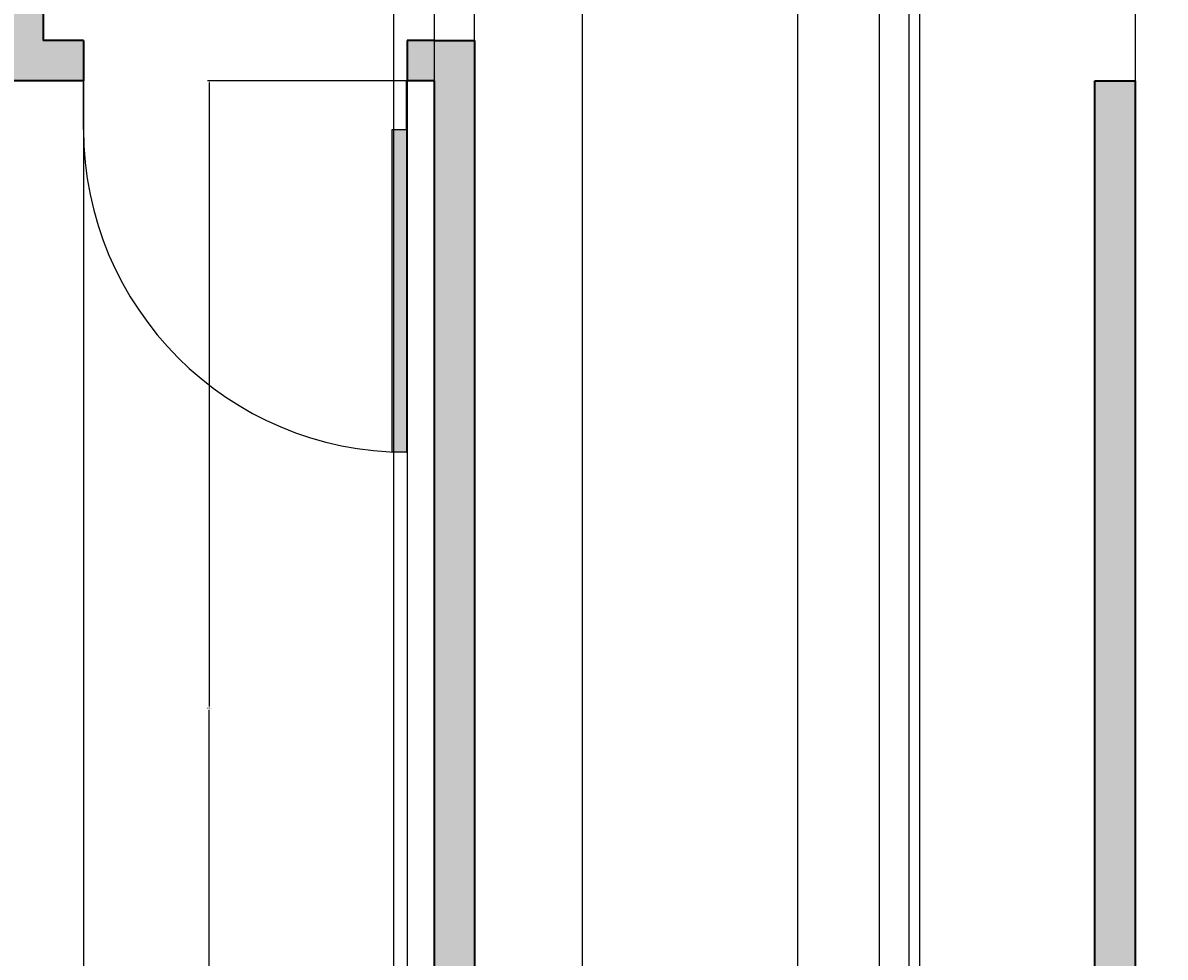
# Model space of a CAD drawing. Units: inches. Extents: x 1434 to 1845, y 1483 to 2014.
# Tile 3 of 11: x 1571 to 1698, y 1633 to 1737. Entities that reach past the tile are written whole.
import ezdxf

# ---------------------------------------------------------------- set-up
doc = ezdxf.new("R2010")
doc.units = ezdxf.units.IN
for name, color, linetype, lineweight in [('A-ANNO-DIMS', 2, 'Continuous', 18), ('A-DOOR', 3, 'Continuous', 25), ('A-WALL', 7, 'Continuous', 35), ('A-WALL-PATT', 8, 'Continuous', 13)]:
    doc.layers.add(name, color=color, linetype=linetype, lineweight=lineweight)
doc.layers.add('A-DOOR-PATT', color=39, linetype='Continuous', lineweight=13, true_color=0x58382b)
doc.styles.get("Standard").update_dxf_attribs({"font": 'arial.ttf'})
doc.dimstyles.get("Standard").update_dxf_attribs({"dimtxt": 0.18, "dimasz": 0.18, "dimexe": 0.18, "dimexo": 0.0625, "dimgap": 0.09, "dimtad": 0, "dimtih": 1, "dimtoh": 1, "dimdec": 4, "dimzin": 0, "dimdsep": 46, "dimtxsty": 'Standard', "dimcen": 0.09, "dimadec": 0, "dimazin": 0, "dimtfac": 1, "dimtdec": 4, "dimtofl": 0, "dimtmove": 0, "dimatfit": 3, "dimfxl": 1, "dimtolj": 1, "dimtzin": 0, "dimarcsym": 0})

# ---------------------------------------------------------------- blocks, each defined once
blk = doc.blocks.new('*U4')
for p, q in [((-40, 0), (-40, 6)), ((0, 0), (0, 6))]:
    blk.add_line(p, q)
blk.add_lwpolyline([(0, 0), (0, -40), (-1.75, -40), (-1.75, 0)], close=True)
blk.add_arc((0, 0), 40, 180, 270)
blk = doc.blocks.new('*D56')
at = {"layer": 'A-ANNO-DIMS', "color": 0, "lineweight": -2, "transparency": 16777216}
for p, q in [((1472.97, 1974.79), (1472.97, 1483.15)), ((1612.47, 1974.79), (1612.47, 1483.15)), ((1473.15, 1483.33), (1542.34, 1483.33)), ((1612.29, 1483.33), (1543.11, 1483.33))]:
    blk.add_line(p, q, dxfattribs=at)
at = {"layer": 'A-ANNO-DIMS', "color": 0, "transparency": 16777216}
for points in [[(1473.15, 1483.36), (1473.15, 1483.3), (1472.97, 1483.33)], [(1612.29, 1483.36), (1612.29, 1483.3), (1612.47, 1483.33)]]:
    blk.add_solid(points, dxfattribs=at)
at = {"layer": 'Defpoints', "color": 0, "transparency": 16777216}
for p in [(1472.97, 1974.86), (1612.47, 1974.86), (1612.47, 1483.33)]:
    blk.add_point(p, dxfattribs=at)
at = {"layer": 'A-ANNO-DIMS', "color": 0, "transparency": 16777216, "insert": (1542.72, 1483.33), "char_height": 0.18, "attachment_point": 5}
blk.add_mtext('\\A1;139.5', dxfattribs=at)
blk = doc.blocks.new('*D57')
at = {"layer": 'A-ANNO-DIMS', "color": 0, "lineweight": -2, "transparency": 16777216}
for p, q in [((1616.97, 1974.79), (1616.97, 1483.15)), ((1666.47, 1974.79), (1666.47, 1483.15)), ((1617.15, 1483.33), (1641.4, 1483.33)), ((1666.29, 1483.33), (1642.05, 1483.33))]:
    blk.add_line(p, q, dxfattribs=at)
at = {"layer": 'A-ANNO-DIMS', "color": 0, "transparency": 16777216}
for points in [[(1617.15, 1483.36), (1617.15, 1483.3), (1616.97, 1483.33)], [(1666.29, 1483.36), (1666.29, 1483.3), (1666.47, 1483.33)]]:
    blk.add_solid(points, dxfattribs=at)
at = {"layer": 'Defpoints', "color": 0, "transparency": 16777216}
for p in [(1616.97, 1974.86), (1666.47, 1974.86), (1666.47, 1483.33)]:
    blk.add_point(p, dxfattribs=at)
at = {"layer": 'A-ANNO-DIMS', "color": 0, "transparency": 16777216, "insert": (1641.72, 1483.33), "char_height": 0.18, "attachment_point": 5}
blk.add_mtext('\\A1;49.5', dxfattribs=at)
blk = doc.blocks.new('*D58')
at = {"layer": 'A-ANNO-DIMS', "color": 0, "lineweight": -2, "transparency": 16777216}
for p, q in [((1670.97, 1974.79), (1670.97, 1483.15)), ((1810.47, 1974.79), (1810.47, 1483.15)), ((1671.15, 1483.33), (1740.34, 1483.33)), ((1810.29, 1483.33), (1741.11, 1483.33))]:
    blk.add_line(p, q, dxfattribs=at)
at = {"layer": 'A-ANNO-DIMS', "color": 0, "transparency": 16777216}
for points in [[(1671.15, 1483.36), (1671.15, 1483.3), (1670.97, 1483.33)], [(1810.29, 1483.36), (1810.29, 1483.3), (1810.47, 1483.33)]]:
    blk.add_solid(points, dxfattribs=at)
at = {"layer": 'Defpoints', "color": 0, "transparency": 16777216}
for p in [(1670.97, 1974.86), (1810.47, 1974.86), (1810.47, 1483.33)]:
    blk.add_point(p, dxfattribs=at)
at = {"layer": 'A-ANNO-DIMS', "color": 0, "transparency": 16777216, "insert": (1740.72, 1483.33), "char_height": 0.18, "attachment_point": 5}
blk.add_mtext('\\A1;139.5', dxfattribs=at)
blk = doc.blocks.new('*D65')
at = {"layer": 'A-ANNO-DIMS', "color": 0, "lineweight": -2, "transparency": 16777216}
for p, q in [((1616.91, 1730.36), (1591.77, 1730.36)), ((1591.95, 1730.18), (1591.95, 1660.79)), ((1591.95, 1591.04), (1591.95, 1660.42)), ((1616.91, 1590.86), (1591.77, 1590.86))]:
    blk.add_line(p, q, dxfattribs=at)
at = {"layer": 'A-ANNO-DIMS', "color": 0, "transparency": 16777216}
for points in [[(1591.92, 1730.18), (1591.98, 1730.18), (1591.95, 1730.36)], [(1591.92, 1591.04), (1591.98, 1591.04), (1591.95, 1590.86)]]:
    blk.add_solid(points, dxfattribs=at)
at = {"layer": 'Defpoints', "color": 0, "transparency": 16777216}
for p in [(1591.95, 1730.36), (1616.97, 1730.36), (1616.97, 1590.86)]:
    blk.add_point(p, dxfattribs=at)
at = {"layer": 'A-ANNO-DIMS', "color": 0, "transparency": 16777216, "insert": (1591.95, 1660.61), "char_height": 0.18, "attachment_point": 5}
blk.add_mtext('\\A1;139.5', dxfattribs=at)
blk = doc.blocks.new('*D67')
at = {"layer": 'A-ANNO-DIMS', "color": 0, "lineweight": -2, "transparency": 16777216}
for p, q in [((1694.97, 1517.42), (1694.97, 2013.56)), ((1695.15, 2013.38), (1752.34, 2013.38)), ((1810.29, 2013.38), (1753.11, 2013.38)), ((1810.47, 1517.42), (1810.47, 2013.56))]:
    blk.add_line(p, q, dxfattribs=at)
at = {"layer": 'A-ANNO-DIMS', "color": 0, "transparency": 16777216}
for points in [[(1695.15, 2013.41), (1695.15, 2013.35), (1694.97, 2013.38)], [(1810.29, 2013.41), (1810.29, 2013.35), (1810.47, 2013.38)]]:
    blk.add_solid(points, dxfattribs=at)
at = {"layer": 'Defpoints', "color": 0, "transparency": 16777216}
for p in [(1810.47, 2013.38), (1694.97, 1517.36), (1810.47, 1517.36)]:
    blk.add_point(p, dxfattribs=at)
at = {"layer": 'A-ANNO-DIMS', "color": 0, "transparency": 16777216, "insert": (1752.72, 2013.38), "char_height": 0.18, "attachment_point": 5}
blk.add_mtext('\\A1;115.5', dxfattribs=at)
blk = doc.blocks.new('*D71')
at = {"layer": 'A-ANNO-DIMS', "color": 0, "lineweight": -2, "transparency": 16777216}
for p, q in [((1633.47, 1508.42), (1633.47, 2013.56)), ((1633.65, 2013.38), (1651.25, 2013.38)), ((1669.64, 2013.38), (1652.04, 2013.38)), ((1669.82, 1508.42), (1669.82, 2013.56))]:
    blk.add_line(p, q, dxfattribs=at)
at = {"layer": 'A-ANNO-DIMS', "color": 0, "transparency": 16777216}
for points in [[(1633.65, 2013.41), (1633.65, 2013.35), (1633.47, 2013.38)], [(1669.64, 2013.41), (1669.64, 2013.35), (1669.82, 2013.38)]]:
    blk.add_solid(points, dxfattribs=at)
at = {"layer": 'Defpoints', "color": 0, "transparency": 16777216}
for p in [(1669.82, 2013.38), (1633.47, 1508.36), (1669.82, 1508.36)]:
    blk.add_point(p, dxfattribs=at)
at = {"layer": 'A-ANNO-DIMS', "color": 0, "transparency": 16777216, "insert": (1651.65, 2013.38), "char_height": 0.18, "attachment_point": 5}
blk.add_mtext('\\A1;36.35', dxfattribs=at)
blk = doc.blocks.new('*D72')
at = {"layer": 'A-ANNO-DIMS', "color": 0, "lineweight": -2, "transparency": 16777216}
for p, q in [((1621.47, 1517.42), (1621.47, 2013.56)), ((1621.65, 2013.38), (1627.26, 2013.38)), ((1633.29, 2013.38), (1627.68, 2013.38)), ((1633.47, 1517.42), (1633.47, 2013.56))]:
    blk.add_line(p, q, dxfattribs=at)
at = {"layer": 'A-ANNO-DIMS', "color": 0, "transparency": 16777216}
for points in [[(1621.65, 2013.41), (1621.65, 2013.35), (1621.47, 2013.38)], [(1633.29, 2013.41), (1633.29, 2013.35), (1633.47, 2013.38)]]:
    blk.add_solid(points, dxfattribs=at)
at = {"layer": 'Defpoints', "color": 0, "transparency": 16777216}
for p in [(1633.47, 2013.38), (1621.47, 1517.36), (1633.47, 1517.36)]:
    blk.add_point(p, dxfattribs=at)
at = {"layer": 'A-ANNO-DIMS', "color": 0, "transparency": 16777216, "insert": (1627.47, 2013.38), "char_height": 0.18, "attachment_point": 5}
blk.add_mtext('\\A1;12', dxfattribs=at)
blk = doc.blocks.new('*D73')
at = {"layer": 'A-ANNO-DIMS', "color": 0, "lineweight": -2, "transparency": 16777216}
for p, q in [((1577.97, 1730.29), (1577.97, 1483.15)), ((1613.97, 1730.29), (1613.97, 1483.15)), ((1578.15, 1483.33), (1595.76, 1483.33)), ((1613.79, 1483.33), (1596.19, 1483.33))]:
    blk.add_line(p, q, dxfattribs=at)
at = {"layer": 'A-ANNO-DIMS', "color": 0, "transparency": 16777216}
for points in [[(1578.15, 1483.36), (1578.15, 1483.3), (1577.97, 1483.33)], [(1613.79, 1483.36), (1613.79, 1483.3), (1613.97, 1483.33)]]:
    blk.add_solid(points, dxfattribs=at)
at = {"layer": 'Defpoints', "color": 0, "transparency": 16777216}
for p in [(1577.97, 1730.36), (1613.97, 1730.36), (1613.97, 1483.33)]:
    blk.add_point(p, dxfattribs=at)
at = {"layer": 'A-ANNO-DIMS', "color": 0, "transparency": 16777216, "insert": (1595.97, 1483.33), "char_height": 0.18, "attachment_point": 5}
blk.add_mtext('\\A1;36', dxfattribs=at)
blk = doc.blocks.new('*D81')
at = {"layer": 'A-ANNO-DIMS', "color": 0, "lineweight": -2, "transparency": 16777216}
for p, q in [((1690.47, 1730.29), (1690.47, 1483.15)), ((1694.97, 1730.29), (1694.97, 1483.15)), ((1690.65, 1483.33), (1692.47, 1483.33)), ((1694.79, 1483.33), (1692.98, 1483.33))]:
    blk.add_line(p, q, dxfattribs=at)
at = {"layer": 'A-ANNO-DIMS', "color": 0, "transparency": 16777216}
for points in [[(1690.65, 1483.36), (1690.65, 1483.3), (1690.47, 1483.33)], [(1694.79, 1483.36), (1694.79, 1483.3), (1694.97, 1483.33)]]:
    blk.add_solid(points, dxfattribs=at)
at = {"layer": 'Defpoints', "color": 0, "transparency": 16777216}
for p in [(1690.47, 1730.36), (1694.97, 1730.36), (1694.97, 1483.33)]:
    blk.add_point(p, dxfattribs=at)
at = {"layer": 'A-ANNO-DIMS', "color": 0, "transparency": 16777216, "insert": (1692.72, 1483.33), "char_height": 0.18, "attachment_point": 5}
blk.add_mtext('\\A1;4.5', dxfattribs=at)
blk = doc.blocks.new('*D86')
at = {"layer": 'A-ANNO-DIMS', "color": 0, "lineweight": -2, "transparency": 16777216}
for p, q in [((1657.38, 1854.66), (1657.38, 1483.15)), ((1666.47, 1854.79), (1666.47, 1483.15)), ((1657.56, 1483.33), (1661.53, 1483.33)), ((1666.29, 1483.33), (1662.32, 1483.33))]:
    blk.add_line(p, q, dxfattribs=at)
at = {"layer": 'A-ANNO-DIMS', "color": 0, "transparency": 16777216}
for points in [[(1657.56, 1483.36), (1657.56, 1483.3), (1657.38, 1483.33)], [(1666.29, 1483.36), (1666.29, 1483.3), (1666.47, 1483.33)]]:
    blk.add_solid(points, dxfattribs=at)
at = {"layer": 'Defpoints', "color": 0, "transparency": 16777216}
for p in [(1657.38, 1854.72), (1666.47, 1854.86), (1657.38, 1483.33)]:
    blk.add_point(p, dxfattribs=at)
at = {"layer": 'A-ANNO-DIMS', "color": 0, "transparency": 16777216, "insert": (1661.93, 1483.33), "char_height": 0.18, "attachment_point": 5}
blk.add_mtext('\\A1;9.096', dxfattribs=at)

msp = doc.modelspace()

# ---------------------------------------------------------------- hatches: boundary and pattern name
at = {"layer": 'A-DOOR-PATT'}
h = msp.add_hatch(color=256, dxfattribs=at)
h.dxf.hatch_style = 1
h.paths.add_polyline_path([(1611.5864, 1583.2737), (1575.6681, 1583.2737, 0.01094143), (1575.7025, 1581.7022), (1611.5864, 1581.7022)])
h.paths.add_polyline_path([(1621.4742, 1547.3553), (1616.9742, 1547.3553), (1616.9742, 1544.3553), (1621.4742, 1544.3553)])
h.paths.add_polyline_path([(1635.0456, 1558.627, 0.01094143), (1633.4742, 1558.6614), (1633.4742, 1522.7431), (1635.0456, 1522.7431)])
h.paths.add_polyline_path([(1633.4742, 1517.3553), (1630.4742, 1517.3553), (1630.4742, 1508.3553), (1633.4742, 1508.3553)])
h.paths.add_polyline_path([(1672.8212, 1517.3553), (1669.8212, 1517.3553), (1669.8212, 1508.3553), (1672.8212, 1508.3553)])
h.paths.add_polyline_path([(1613.8925, 1724.9676), (1612.3211, 1724.9676), (1612.3211, 1689.0836, 0.01094143), (1613.8925, 1689.0492)])
h.paths.add_polyline_path([(1789.3925, 1684.9726), (1753.4742, 1684.9726), (1753.4742, 1683.4011), (1789.3925, 1683.4011)])
h.paths.add_polyline_path([(1792.4742, 1679.5848), (1789.4742, 1679.5848), (1789.4742, 1675.0848), (1792.4742, 1675.0848)])
h.paths.add_polyline_path([(1563.5864, 1851.7737), (1527.6681, 1851.7737, 0.01094143), (1527.7025, 1850.2022), (1563.5864, 1850.2022)])
h.paths.add_polyline_path([(1609.3925, 1900.6614, 0.01094143), (1607.8211, 1900.627), (1607.8211, 1864.7431), (1609.3925, 1864.7431)])
h.paths.add_polyline_path([(1675.5456, 1900.627, 0.01094143), (1673.9742, 1900.6614), (1673.9742, 1864.7431), (1675.5456, 1864.7431)])
h.paths.add_polyline_path([(1751.2803, 1851.8553), (1715.3619, 1851.8553), (1715.3619, 1850.2839), (1751.2459, 1850.2839, 0.01094143)])
at = {"layer": 'A-WALL-PATT'}
h = msp.add_hatch(color=256, dxfattribs=at)
h.dxf.hatch_style = 1
h.paths.add_polyline_path([(1472.9742, 1730.3553), (1577.9742, 1730.3553), (1577.9742, 1734.8553), (1573.4742, 1734.8553), (1573.4742, 1815.8553), (1568.9742, 1815.8553), (1568.9742, 1734.8553), (1472.9742, 1734.8553), (1472.9742, 1770.1951), (1459.9742, 1770.1951), (1459.9742, 1782.1951), (1459.9742, 1818.1951), (1472.9742, 1818.1951), (1472.9742, 1854.8553), (1568.9742, 1854.8553), (1568.9742, 1851.8553), (1573.4742, 1851.8553), (1573.4742, 1854.8553), (1573.4742, 1859.3553), (1472.9742, 1859.3553), (1472.9742, 1899.9369), (1459.9742, 1899.9369), (1459.9742, 1911.9369), (1459.9742, 1947.9369), (1472.9742, 1947.9369), (1472.9742, 1974.8553), (1513.9785, 1974.8553), (1513.9785, 1987.8553), (1561.9785, 1987.8553), (1561.9785, 1974.8553), (1612.4742, 1974.8553), (1612.4742, 1859.3553), (1609.4742, 1859.3553), (1609.4742, 1854.8553), (1616.9742, 1854.8553), (1616.9742, 1910.3553), (1625.153, 1910.3553), (1625.153, 1914.8553), (1616.9742, 1914.8553), (1616.9742, 1988.3553), (1459.4742, 1988.3553), (1459.4742, 1508.3553), (1630.4742, 1508.3553), (1630.4742, 1517.3553), (1472.9742, 1517.3553), (1472.9742, 1586.3553), (1616.9742, 1586.3553), (1616.9742, 1583.3553), (1621.4742, 1583.3553), (1621.4742, 1586.3553), (1621.4742, 1734.8553), (1616.9742, 1734.8553), (1613.9742, 1734.8553), (1613.9742, 1730.3553), (1616.9742, 1730.3553), (1616.9742, 1590.8553), (1472.9742, 1590.8553), (1472.9742, 1635.7299), (1459.9742, 1635.7299), (1459.9742, 1647.7299), (1459.9742, 1683.7299), (1472.9742, 1683.7299)])
h.paths.add_polyline_path([(1819.4742, 1773.1667), (1810.4742, 1773.1667), (1810.4742, 1734.8553), (1714.4742, 1734.8553), (1714.4742, 1815.8553), (1709.9742, 1815.8553), (1709.9742, 1730.3553), (1745.9742, 1730.3553), (1745.9742, 1675.0848), (1753.4742, 1675.0848), (1753.4742, 1679.5848), (1750.4742, 1679.5848), (1750.4742, 1730.3553), (1810.4742, 1730.3553), (1810.4742, 1679.5848), (1792.4742, 1679.5848), (1792.4742, 1675.0848), (1810.4742, 1675.0848), (1810.4742, 1517.3553), (1775.1129, 1517.3553), (1775.1129, 1508.3553), (1819.4742, 1508.3553)])
h.paths.add_polyline_path([(1739.1129, 1517.3553), (1694.9742, 1517.3553), (1694.9742, 1730.3553), (1690.4742, 1730.3553), (1690.4742, 1517.3553), (1678.4742, 1517.3553), (1675.4742, 1517.3553), (1672.8212, 1517.3553), (1672.8212, 1508.3553), (1678.4742, 1508.3553), (1739.1129, 1508.3553)])
h.paths.add_polyline_path([(1735.6549, 1987.8553), (1783.6549, 1987.8553), (1783.6549, 1974.8553), (1810.4742, 1974.8553), (1810.4742, 1859.3553), (1709.9742, 1859.3553), (1709.9742, 1854.8553), (1709.9742, 1851.8553), (1714.4742, 1851.8553), (1714.4742, 1854.8553), (1810.4742, 1854.8553), (1810.4742, 1809.1667), (1819.4742, 1809.1667), (1819.4742, 1988.3553), (1666.4742, 1988.3553), (1666.4742, 1914.8553), (1661.1087, 1914.8553), (1661.1087, 1910.3553), (1666.4742, 1910.3553), (1666.4742, 1854.8553), (1673.9742, 1854.8553), (1673.9742, 1859.3553), (1670.9742, 1859.3553), (1670.9742, 1974.8553), (1735.6549, 1974.8553)])

# ---------------------------------------------------------------- linework, layer by layer
at = {"layer": 'A-WALL'}
for p, q in [((1573.4742, 1815.8553), (1573.4742, 1734.8553)), ((1577.9742, 1734.8553), (1573.4742, 1734.8553)), ((1577.9742, 1734.8553), (1577.9742, 1730.3553)), ((1616.9742, 1734.8553), (1613.9742, 1734.8553)), ((1613.9742, 1734.8553), (1613.9742, 1730.3553)), ((1616.9742, 1734.8553), (1621.4742, 1734.8553)), ((1621.4742, 1734.8553), (1621.4742, 1586.3553)), ((1577.9742, 1730.3553), (1472.9742, 1730.3553)), ((1616.9742, 1730.3553), (1613.9742, 1730.3553)), ((1616.9742, 1730.3553), (1616.9742, 1590.8553)), ((1690.4742, 1517.3553), (1690.4742, 1730.3553)), ((1690.4742, 1730.3553), (1694.9742, 1730.3553)), ((1694.9742, 1517.3553), (1694.9742, 1730.3553))]:
    msp.add_line(p, q, dxfattribs=at)

# ---------------------------------------------------------------- block references
at = {"layer": 'A-DOOR', "xscale": 0.8979587755198419, "yscale": 0.8979587755198419, "zscale": 0.8979587755198419}
msp.add_blockref('*U4', (1613.8925, 1724.9676), dxfattribs=at)

# ---------------------------------------------------------------- dimensions: what is measured, and where the dimension line sits
at = {"layer": 'A-ANNO-DIMS'}
for base, p1, p2, override, picture, middle in [((1633.4742, 2013.3803), (1621.4742, 1517.3553), (1633.4742, 1517.3553), {"dimdec": 0, "dimlfac": 1, "dimrnd": 0, "dimzin": 0, "dimdsep": 46, "dimlunit": 2}, '*D72', (1627.4742, 2013.3803)), ((1669.8212, 2013.3803), (1633.4742, 1508.3553), (1669.8212, 1508.3553), {"dimdec": 2, "dimlfac": 1, "dimrnd": 0, "dimzin": 0, "dimdsep": 46, "dimlunit": 2}, '*D71', (1651.6477, 2013.3803)), ((1810.4742, 2013.3803), (1694.9742, 1517.3553), (1810.4742, 1517.3553), {"dimdec": 1, "dimlfac": 1, "dimrnd": 0, "dimzin": 0, "dimdsep": 46, "dimlunit": 2}, '*D67', (1752.7242, 2013.3803)), ((1612.4742, 1483.3303), (1472.9742, 1974.8553), (1612.4742, 1974.8553), {"dimdec": 1, "dimlfac": 1, "dimrnd": 0, "dimzin": 0, "dimdsep": 46, "dimlunit": 2}, '*D56', (1542.7242, 1483.3303)), ((1666.4742, 1483.3303), (1616.9742, 1974.8553), (1666.4742, 1974.8553), {"dimdec": 1, "dimlfac": 1, "dimrnd": 0, "dimzin": 0, "dimdsep": 46, "dimlunit": 2}, '*D57', (1641.7242, 1483.3303)), ((1810.4742, 1483.3303), (1670.9742, 1974.8553), (1810.4742, 1974.8553), {"dimdec": 1, "dimlfac": 1, "dimrnd": 0, "dimzin": 0, "dimdsep": 46, "dimlunit": 2}, '*D58', (1740.7242, 1483.3303)), ((1657.3781, 1483.3303), (1666.4742, 1854.8553), (1657.3781, 1854.7205), {"dimdec": 3, "dimlfac": 1, "dimrnd": 0, "dimzin": 0, "dimdsep": 46, "dimlunit": 2}, '*D86', (1661.9261, 1483.3303)), ((1613.9742, 1483.3303), (1577.9742, 1730.3553), (1613.9742, 1730.3553), {"dimdec": 0, "dimlfac": 1, "dimrnd": 0, "dimzin": 0, "dimdsep": 46, "dimlunit": 2}, '*D73', (1595.9742, 1483.3303)), ((1694.9742, 1483.3303), (1690.4742, 1730.3553), (1694.9742, 1730.3553), {"dimdec": 1, "dimlfac": 1, "dimrnd": 0, "dimzin": 0, "dimdsep": 46, "dimlunit": 2}, '*D81', (1692.7242, 1483.3303))]:
    dim = msp.add_linear_dim(base=base, p1=p1, p2=p2, dimstyle='Standard', override=override, dxfattribs=at)
    dim.commit()
    dim.dimension.update_dxf_attribs({"geometry": picture, "text_midpoint": middle})
dim = msp.add_linear_dim(base=(1591.9492, 1730.3553), p1=(1616.9742, 1590.8553), p2=(1616.9742, 1730.3553), angle=90, dimstyle='Standard', override={"dimdec": 1, "dimlfac": 1, "dimrnd": 0, "dimzin": 0, "dimdsep": 46, "dimlunit": 2}, dxfattribs=at)
dim.commit()
dim.dimension.update_dxf_attribs({"geometry": '*D65', "text_midpoint": (1591.9492, 1660.6053)})

doc.saveas('drawing.dxf')
